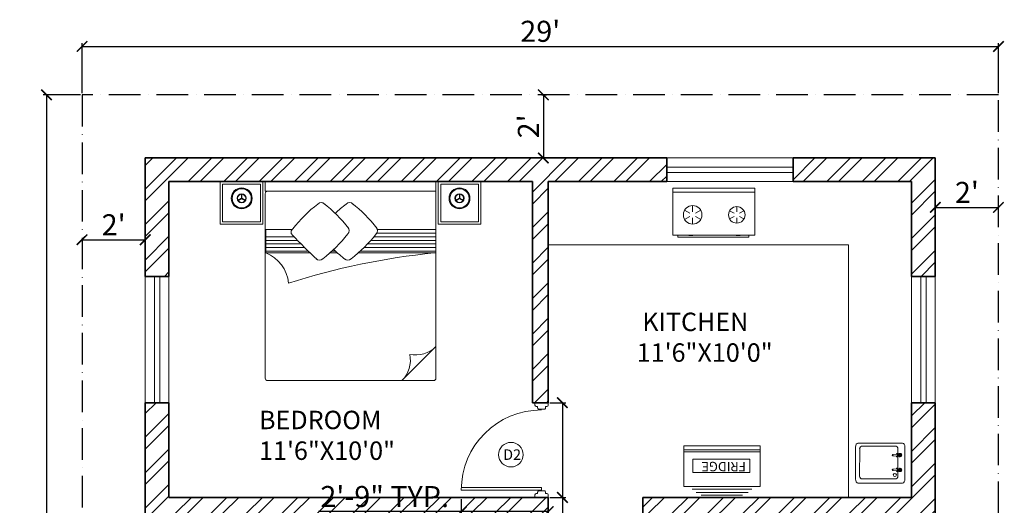
# Model space of a CAD drawing. Units: inches. Extents: x -15 to 1053, y -1 to 793.
# Tile 3 of 8: x 21 to 395, y 609 to 793. Entities that reach past the tile are written whole.
import ezdxf

# ---------------------------------------------------------------- set-up
doc = ezdxf.new("R2010")
doc.units = ezdxf.units.IN
doc.linetypes.add('ACAD_ISO10W100', pattern=[18, 12, -3, 0, -3])
for name, color, linetype, lineweight in [('00 FURNITURE', 15, 'Continuous', 15), ('A-ANNO-DIMS', 2, 'Continuous', 18), ('A-ANNO-TEXT', 7, 'Continuous', 18), ('A-AREA-IDEN', 7, 'Continuous', 18), ('A-DOOR', 4, 'Continuous', 18), ('A-FLOR-CASE', 5, 'Continuous', 18), ('A-FLOR-FIXT', 8, 'Continuous', 13), ('A-FURN', 8, 'Continuous', 13), ('A-GLAZ', 4, 'Continuous', 18), ('A-WALL', 7, 'Continuous', 35), ('A-WALL-PATT', 8, 'Continuous', 13), ('C-PROP', 1, 'ACAD_ISO10W100', 25)]:
    doc.layers.add(name, color=color, linetype=linetype, lineweight=lineweight)
doc.layers.add('FURN3D', color=229, linetype='Continuous', lineweight=5, true_color=0x4a3f41)
doc.layers.add('furniture', color=253, linetype='Continuous', lineweight=9, transparency=0.4)
doc.styles.add('1-100DIM', font='txt', dxfattribs={"height": 0.3})
doc.styles.get("Standard").update_dxf_attribs({"font": 'arial.ttf'})
doc.dimstyles.new('ISO-25', dxfattribs={"dimtxt": 8, "dimasz": 4, "dimexe": 1.25, "dimexo": 0.625, "dimtad": 1, "dimdec": 0, "dimlunit": 4, "dimtxsty": 'Standard', "dimblk": 'ARCHTICK', "dimcen": 3, "dimadec": 0, "dimazin": 0, "dimtfac": 1, "dimtdec": 0, "dimtmove": 0, "dimatfit": 3, "dimldrblk": 'ARCHTICK', "dimfxl": 1, "dimarcsym": 0})

# ---------------------------------------------------------------- blocks, each defined once
blk = doc.blocks.new('A$C21540130')
at = {"layer": 'FURN3D'}
for p, q in [((1.57, 0), (1.57, 31.11)), ((9.61, 25.31), (8.63, 27.01)), ((10.79, 25.31), (11.77, 27.01)), ((9.02, 24.29, -27.54), (7.06, 24.29, -27.54)), ((9.61, 23.27), (8.63, 21.57)), ((10.79, 23.27), (11.77, 21.57)), ((11.38, 24.29, -27.54), (13.34, 24.29, -27.54)), ((9.02, 7.54), (6.67, 7.54)), ((9.61, 8.56), (8.43, 10.6)), ((10.79, 8.56), (11.97, 10.6)), ((11.38, 7.54), (13.73, 7.54)), ((9.61, 6.52), (8.43, 4.48)), ((10.79, 6.52), (11.97, 4.48))]:
    blk.add_line(p, q, dxfattribs=at)
for points in [[(0, 0), (0, 31.11), (17.9, 31.11), (17.9, 0)], [(18.68, 1.96), (18.68, 28.83), (17.9, 28.83), (17.9, 1.96)]]:
    blk.add_lwpolyline(points, close=True, dxfattribs=at)
for centre, radius in [((10.2, 24.29), 3.14), ((10.2, 7.54), 3.53)]:
    blk.add_circle(centre, radius, dxfattribs=at)
for points in [[(17.9, 24.03), (18.29, 24.03), (17.9, 25.6), (18.29, 25.6)], [(17.9, 6.05), (18.29, 6.05), (17.9, 7.62), (18.29, 7.62)]]:
    blk.add_solid(points, dxfattribs=at)
blk = doc.blocks.new('A$C03CC5C65')
at = {"layer": 'FURN3D'}
for p, q in [((1.56, 18.72, -49.92), (13.66, 18.72, -49.92)), ((0, 0.9, -49.92), (0, 17.82, -49.92)), ((0, 0.9, -29.27), (0, 17.82, -48.65)), ((0, 17.82, -29.27), (0, 0.9, -48.65)), ((4.37, 16.77, -25.9), (4.37, 16.84, -25.9)), ((4.37, 16.77, -25.9), (4.73, 16.4, -25.9)), ((4.37, 15.7, -25.9), (4.73, 16.12, -25.9)), ((4.37, 15.64, -25.9), (4.73, 16.06, -25.9)), ((4.37, 15.64, -25.9), (4.37, 15.7, -25.9)), ((4.48, 16.95, -25.9), (4.87, 16.59, -25.9)), ((4.48, 16.89, -25.9), (4.48, 16.95, -25.9)), ((4.48, 16.89, -25.9), (4.87, 16.52, -25.9)), ((4.48, 15.53, -25.9), (4.87, 15.89, -25.9)), ((4.63, 16.87, -25.9), (4.63, 16.8, -25.9)), ((4.63, 15.67, -25.9), (4.68, 15.67, -25.9)), ((4.63, 15.67), (4.68, 15.67)), ((4.64, 16.49, -25.9), (4.66, 16.05, -25.9)), ((4.83, 16.98, -25.9), (4.68, 16.76, -25.9)), ((4.68, 15.71, -25.9), (4.75, 14.17, -25.9)), ((4.87, 16.91, -25.9), (4.73, 16.71, -25.9)), ((5.24, 16.98, -25.9), (4.83, 16.98, -25.9)), ((4.87, 16.91, -25.9), (4.83, 16.98, -25.9)), ((5.21, 16.91, -25.9), (4.87, 16.91, -25.9)), ((5.21, 16.91, -25.9), (5.24, 16.98, -25.9)), ((5.6, 16.95, -25.9), (5.21, 16.59, -25.9)), ((5.21, 16.91, -25.9), (5.34, 16.71, -25.9)), ((5.6, 16.88, -25.9), (5.21, 16.52, -25.9)), ((5.6, 15.52, -25.9), (5.21, 15.89, -25.9)), ((5.24, 16.98, -25.9), (5.39, 16.76, -25.9)), ((5.39, 15.71, -25.9), (5.32, 14.17, -25.9)), ((5.71, 16.77, -25.9), (5.35, 16.4, -25.9)), ((5.71, 15.7, -25.9), (5.35, 16.12, -25.9)), ((5.71, 15.64, -25.9), (5.35, 16.06, -25.9)), ((5.39, 15.67, -25.9), (5.44, 15.67, -25.9)), ((5.39, 15.67), (5.44, 15.67)), ((5.43, 16.49, -25.9), (5.41, 16.05, -25.9)), ((5.44, 16.87, -25.9), (5.44, 16.8, -25.9)), ((5.6, 16.95, -25.9), (5.6, 16.88, -25.9)), ((5.6, 16.95, -25.9), (5.6, 16.88, -25.9)), ((5.71, 16.77, -25.9), (5.71, 16.83, -25.9)), ((5.71, 15.64, -25.9), (5.71, 15.7, -25.9)), ((9.98, 15.69, -25.9), (10.34, 16.11, -25.9)), ((9.98, 15.63, -25.9), (10.34, 16.05, -25.9)), ((9.98, 15.63, -25.9), (9.98, 15.69, -25.9)), ((9.99, 16.76, -25.9), (9.99, 16.83, -25.9)), ((9.99, 16.76, -25.9), (10.34, 16.39, -25.9)), ((10.09, 16.94, -25.9), (10.48, 16.58, -25.9)), ((10.09, 16.88, -25.9), (10.09, 16.94, -25.9)), ((10.09, 16.88, -25.9), (10.48, 16.51, -25.9)), ((10.09, 15.52, -25.9), (10.48, 15.88, -25.9)), ((10.25, 16.86, -25.9), (10.25, 16.8, -25.9)), ((10.25, 15.66, -25.9), (10.3, 15.66, -25.9)), ((10.25, 15.66), (10.3, 15.66)), ((10.26, 16.47, -25.9), (10.28, 16.03, -25.9)), ((10.45, 16.97, -25.9), (10.3, 16.75, -25.9)), ((10.3, 15.7, -25.9), (10.37, 14.16, -25.9)), ((10.49, 16.9, -25.9), (10.35, 16.7, -25.9)), ((10.86, 16.97, -25.9), (10.45, 16.97, -25.9)), ((10.49, 16.9, -25.9), (10.45, 16.97, -25.9)), ((10.82, 16.9, -25.9), (10.49, 16.9, -25.9)), ((10.82, 16.9, -25.9), (10.86, 16.97, -25.9)), ((11.22, 16.94, -25.9), (10.82, 16.58, -25.9)), ((10.82, 16.9, -25.9), (10.96, 16.7, -25.9)), ((11.22, 16.88, -25.9), (10.82, 16.51, -25.9)), ((11.21, 15.51, -25.9), (10.82, 15.88, -25.9)), ((10.86, 16.97, -25.9), (11.01, 16.75, -25.9)), ((11.01, 15.7, -25.9), (10.93, 14.16, -25.9)), ((11.32, 16.76, -25.9), (10.96, 16.39, -25.9)), ((11.32, 15.69, -25.9), (10.96, 16.11, -25.9)), ((11.32, 15.63, -25.9), (10.96, 16.05, -25.9)), ((11.01, 15.66, -25.9), (11.06, 15.66, -25.9)), ((11.01, 15.66), (11.06, 15.66)), ((11.05, 16.47, -25.9), (11.03, 16.03, -25.9)), ((11.06, 16.86, -25.9), (11.06, 16.8, -25.9)), ((11.22, 16.94, -25.9), (11.22, 16.88, -25.9)), ((11.22, 16.94, -25.9), (11.22, 16.88, -25.9)), ((11.32, 16.76, -25.9), (11.32, 16.83, -25.9)), ((11.32, 15.63, -25.9), (11.32, 15.69, -25.9)), ((15.22, 0.9, -29.27), (15.22, 17.82, -48.65)), ((15.22, 17.82, -29.27), (15.22, 0.9, -48.65)), ((1.56, 0, -28), (13.66, 0, -28))]:
    blk.add_line(p, q, dxfattribs=at)
at = {"layer": 'FURN3D', "elevation": -25.9}
for points in [[(1.61, 15.14), (1.62, 2.5)], [(4.66, 16.1), (2.57, 16.1)], [(10.28, 16.11), (5.41, 16.1)], [(13.12, 16.11), (11.03, 16.11)], [(14.1, 2.52), (14.09, 15.15)], [(2.58, 1.55), (13.13, 1.56)]]:
    blk.add_lwpolyline(points, dxfattribs=at)
at = {"layer": 'FURN3D'}
for centre, radius in [((3.1, 14.9, -25.9), 0.593), ((5.04, 16.22, -25.9), 0.218), ((5.04, 16.87), 0.203), ((5.04, 16.87, -25.9), 0.203), ((10.65, 16.22, -25.9), 0.218), ((10.65, 16.86), 0.203), ((10.65, 16.86, -25.9), 0.203)]:
    blk.add_circle(centre, radius, dxfattribs=at)
at = {"layer": 'FURN3D', "extrusion": (0, 0.814703, 0.579878)}
for centre, start, end in [((-1.56, -49.97, -13.7), 270, 0), ((-13.66, -49.97, -13.7), 180, 270), ((-1.56, -24.37, -16.24), 0, 90), ((-13.66, -24.37, -16.24), 90, 180)]:
    blk.add_arc(centre, 1.56, start, end, dxfattribs=at)
at = {"layer": 'FURN3D', "extrusion": (2.9e-15, -0.814703, 0.579878)}
for centre, start, end in [((1.56, -13.52, -31.49), 90, 180), ((1.56, -39.11, -28.95), 180, 270)]:
    blk.add_arc(centre, 1.56, start, end, dxfattribs=at)
at = {"layer": 'FURN3D', "extrusion": (-2.9e-15, -0.814703, 0.579878)}
for centre, start, end in [((13.66, -13.52, -31.49), 0, 90), ((13.66, -39.11, -28.95), 270, 0)]:
    blk.add_arc(centre, 1.56, start, end, dxfattribs=at)
at = {"layer": 'FURN3D'}
for centre, radius, start, end in [((2.6, 15.1, -25.9), 0.997, 88.2299, 182.3676), ((4.6, 16.73, -25.9), 0.252, 118.1078, 154.1122), ((4.6, 16.66, -25.9), 0.252, 118.1078, 154.1122), ((4.6, 15.75, -25.9), 0.252, 205.7141, 241.7184), ((5.04, 16.87, -25.9), 0.655, 359.2227, 180.6036), ((5.04, 16.88, -25.9), 0.655, 190.8582, 233.614), ((5.04, 16.87, -25.9), 0.406, 359.9131, 179.9131), ((4.54, 16.23, -25.9), 0.25, 317.2189, 42.6074), ((4.54, 16.29, -25.9), 0.25, 317.2189, 352.664), ((5.04, 16.6, -25.9), 0.312, 19.462, 160.6639), ((5.04, 16.24, -25.9), 0.218, 356.8132, 183.0131), ((5.04, 16.77, -25.9), 0.25, 227.2092, 312.6171), ((5.04, 16.71, -25.9), 0.25, 227.2092, 312.6171), ((5.04, 15.7, -25.9), 0.25, 47.2092, 132.6171), ((5.04, 16.44, -25.9), 0.187, 40.218, 139.6082), ((5.53, 16.23, -25.9), 0.25, 137.2189, 222.6074), ((5.53, 16.29, -25.9), 0.25, 187.1622, 222.6074), ((5.04, 16.88, -25.9), 0.655, 306.2123, 348.968), ((5.48, 16.72, -25.9), 0.252, 25.7141, 61.7184), ((5.48, 16.66, -25.9), 0.252, 25.7141, 61.7184), ((5.48, 15.75, -25.9), 0.252, 298.1078, 334.1122), ((10.21, 15.74, -25.9), 0.252, 205.7141, 241.7184), ((10.21, 16.72, -25.9), 0.252, 118.1078, 154.1122), ((10.21, 16.65, -25.9), 0.252, 118.1078, 154.1122), ((10.65, 16.86, -25.9), 0.655, 359.2227, 180.6036), ((10.65, 16.86, -25.9), 0.655, 190.8582, 233.614), ((10.65, 16.86, -25.9), 0.406, 359.9131, 179.9131), ((10.16, 16.22, -25.9), 0.25, 317.2189, 42.6074), ((10.16, 16.28, -25.9), 0.25, 317.2189, 352.664), ((10.66, 16.59, -25.9), 0.312, 19.462, 160.6639), ((10.65, 16.23, -25.9), 0.218, 356.8132, 183.0131), ((10.65, 16.7, -25.9), 0.25, 227.2092, 312.6171), ((10.65, 15.69, -25.9), 0.25, 47.2092, 132.6171), ((10.65, 16.76, -25.9), 0.25, 227.2092, 312.6171), ((10.65, 16.44, -25.9), 0.187, 40.218, 139.6082), ((11.15, 16.22, -25.9), 0.25, 137.2189, 222.6074), ((11.15, 16.28, -25.9), 0.25, 187.1622, 222.6074), ((10.65, 16.86, -25.9), 0.655, 306.2123, 348.968), ((11.1, 15.74, -25.9), 0.252, 298.1078, 334.1122), ((11.1, 16.72, -25.9), 0.252, 25.7141, 61.7184), ((11.1, 16.65, -25.9), 0.252, 25.7141, 61.7184), ((13.09, 15.11, -25.9), 0.997, 357.7426, 91.8802), ((5.04, 14.37, -25.9), 0.298, 194.8671, 343.5351), ((5.03, 14.18, -25.9), 0.281, 182.7661, 357.0602), ((10.65, 14.36, -25.9), 0.298, 194.8671, 343.5351), ((10.65, 14.17, -25.9), 0.281, 182.7661, 357.0602), ((2.61, 2.54, -25.9), 0.997, 177.7426, 271.8802), ((13.1, 2.55, -25.9), 0.997, 268.2299, 2.3676)]:
    blk.add_arc(centre, radius, start, end, dxfattribs=at)
blk = doc.blocks.new('RGWTG')
at = {"layer": '00 FURNITURE'}
for p, q in [((578.23, 3473.51), (577.36, 3475.01)), ((578.23, 3473.58), (577.36, 3472.08)), ((578.36, 3473.58), (577.49, 3475.09)), ((578.36, 3473.51), (577.49, 3472)), ((578.29, 3473.62), (580.03, 3473.62)), ((578.29, 3473.47), (580.03, 3473.47)), ((521.93, 3464.58), (509.03, 3451.68)), ((509.03, 3422.63), (509.03, 3463.68)), ((509.93, 3464.58), (566.4, 3464.58)), ((557.53, 3463.84), (557.53, 3464.49)), ((557.53, 3464.49), (566.4, 3464.49)), ((558.2, 3464.49), (558.2, 3435.82)), ((559.57, 3464.49), (559.57, 3437.25)), ((560.94, 3464.49), (560.94, 3438.58)), ((562.3, 3464.49), (562.3, 3439.83)), ((563.67, 3464.49), (563.67, 3440.99)), ((565.04, 3464.49), (565.04, 3442.08)), ((566.4, 3464.58), (580.98, 3464.58)), ((566.4, 3464.49), (566.4, 3442.08)), ((566.4, 3464.49), (566.4, 3463.84)), ((580.98, 3464.58), (580.98, 3416.72)), ((558.2, 3426.48), (558.2, 3425.04)), ((509.03, 3400.68), (509.03, 3422.63)), ((558.2, 3416.13), (558.2, 3399.95)), ((559.57, 3414.75), (559.57, 3399.95)), ((580.98, 3416.72), (580.98, 3400.68)), ((560.94, 3413.39), (560.94, 3399.95)), ((562.3, 3412.04), (562.3, 3399.95)), ((563.67, 3410.72), (563.67, 3399.95)), ((580.08, 3399.78), (509.93, 3399.78)), ((557.53, 3399.95), (557.53, 3400.6)), ((566.4, 3399.95), (557.53, 3399.95)), ((566.4, 3400.6), (566.4, 3399.95)), ((578.23, 3390.78), (577.36, 3392.29)), ((578.36, 3390.86), (577.49, 3392.36)), ((578.23, 3390.86), (577.36, 3389.36)), ((578.36, 3390.78), (577.49, 3389.28)), ((578.29, 3390.9), (580.03, 3390.9)), ((578.29, 3390.74), (580.03, 3390.74))]:
    blk.add_line(p, q, dxfattribs=at)
for points in [[(568.43, 3465.48), (584.63, 3465.48), (584.63, 3481.68), (568.43, 3481.68)], [(569.33, 3466.38), (583.73, 3466.38), (583.73, 3480.78), (569.33, 3480.78)], [(580.98, 3399.78), (584.63, 3399.78), (584.63, 3464.58), (580.98, 3464.58)], [(568.43, 3398.88), (584.63, 3398.88), (584.63, 3382.68), (568.43, 3382.68)], [(569.33, 3397.98), (583.73, 3397.98), (583.73, 3383.58), (569.33, 3383.58)]]:
    blk.add_lwpolyline(points, close=True, dxfattribs=at)
for points in [[(566.52, 3464.49), (557.53, 3464.49), (557.53, 3435.08)], [(557.53, 3427.21), (557.53, 3424.3)], [(557.53, 3416.82), (557.53, 3399.95), (566.4, 3399.95), (566.4, 3409.94)]]:
    blk.add_lwpolyline(points, dxfattribs=at)
for centre, radius in [((578.29, 3473.54), 3.97), ((578.29, 3473.54), 3.63), ((578.29, 3473.54), 1.74), ((578.29, 3473.54), 1.56), ((578.29, 3390.82), 3.97), ((578.29, 3390.82), 3.63), ((578.29, 3390.82), 1.74), ((578.29, 3390.82), 1.56)]:
    blk.add_circle(centre, radius, dxfattribs=at)
for centre, radius, start, end in [((509.93, 3463.68), 0.9, 90, 180), ((529.65, 3456.88), 10.9, 135.0361, 191.9278), ((290.56, 3490.52), 268.3, 342.2214, 354.2925), ((516.73, 3443.97), 10.9, 78.0722, 134.9639), ((598.15, 3399.01), 54.32, 127.931, 142.069), ((566.05, 3440.57), 1.82, 45, 135), ((533.58, 3399.31), 54.32, 37.931, 52.069), ((556.59, 3431.11), 1.82, 135, 225), ((574.84, 3431.77), 1.82, 315, 45), ((597.87, 3463.6), 54.32, 217.931, 224.141), ((598.15, 3388.23), 54.32, 127.931, 142.069), ((566.05, 3429.78), 1.82, 45, 135), ((533.58, 3388.53), 54.32, 37.931, 52.069), ((533.28, 3463.88), 54.32, 316.32, 322.069), ((556.59, 3420.33), 1.82, 135, 225), ((574.84, 3420.99), 1.82, 315, 45), ((765.33, 3619.75), 290.45, 223.6069, 226.2326), ((533.28, 3453.1), 54.32, 307.931, 322.069), ((565.44, 3411.05), 1.47, 225.9674, 326.8337), ((545.02, 3395.29), 13.35, 20.4224, 85.5825), ((509.93, 3400.68), 0.9, 180, 270), ((580.08, 3400.68), 0.9, 270, 0)]:
    blk.add_arc(centre, radius, start, end, dxfattribs=at)
blk = doc.blocks.new('DDD')
at = {"layer": '00 FURNITURE'}
for p, q in [((-12579.77, -15859.53), (-12579.77, -15829.05)), ((-12578.77, -15859.53), (-12578.77, -15829.03)), ((-12612.02, -15857.03), (-12612.02, -15862.03)), ((-12611.02, -15857.03), (-12612.02, -15857.03)), ((-12610.52, -15858.03), (-12610.52, -15857.53)), ((-12578.77, -15859.53), (-12579.77, -15859.53)), ((-12577.52, -15858.03), (-12577.52, -15857.53)), ((-12577.02, -15857.03), (-12576.02, -15857.03)), ((-12576.02, -15857.03), (-12576.02, -15862.03)), ((-12612.02, -15862.03), (-12611.02, -15862.03)), ((-12610.52, -15861.53), (-12610.52, -15861.03)), ((-12577.52, -15861.53), (-12577.52, -15861.03)), ((-12576.02, -15862.03), (-12577.02, -15862.03))]:
    blk.add_line(p, q, dxfattribs=at)
for points in [[(-12610.52, -15861.03), (-12610.02, -15861.03, 0.414214), (-12609.52, -15860.53), (-12609.52, -15858.53, 0.414214), (-12610.02, -15858.03), (-12610.52, -15858.03)], [(-12577.52, -15861.03), (-12578.02, -15861.03, -0.414214), (-12578.52, -15860.53), (-12578.52, -15858.53, -0.414214), (-12578.02, -15858.03), (-12577.52, -15858.03)]]:
    blk.add_lwpolyline(points, format="xyb", dxfattribs=at)
for centre, radius, start, end in [((-12578.77, -15859.53), 30.5, 90, 180), ((-12611.02, -15857.53), 0.5, 0, 90), ((-12577.02, -15857.53), 0.5, 90, 180), ((-12611.02, -15861.53), 0.5, 270, 0), ((-12577.02, -15861.53), 0.5, 180, 270)]:
    blk.add_arc(centre, radius, start, end, dxfattribs=at)
blk = doc.blocks.new('A$C5BBA3387')
at = {"layer": 'furniture'}
for p, q in [((16.49, 29.07), (16.49, 0)), ((17.22, 29.07), (17.22, 0)), ((0, 22.44), (0, 6.75)), ((1.08, 24.37), (1.08, 4.58)), ((2.29, 25.81), (2.29, 3.26))]:
    blk.add_line(p, q, dxfattribs=at)
for points in [[(18.78, 29.07), (18.78, 0), (3.37, 0), (3.37, 29.07)], [(8.63, 4.02), (8.63, 25.56), (13.78, 25.56), (13.78, 4.02)]]:
    blk.add_lwpolyline(points, close=True, dxfattribs=at)
at = {"layer": 'furniture', "insert": (9.12, 5.47), "char_height": 3.589, "width": 57.8029, "attachment_point": 1, "rotation": 90}
blk.add_mtext('FRIDGE', dxfattribs=at)
blk = doc.blocks.new('_ArchTick')
at = {"color": 0, "linetype": 'ByBlock', "const_width": 0.15}
blk.add_lwpolyline([(-0.5, -0.5), (0.5, 0.5)], dxfattribs=at)
blk = doc.blocks.new('*D16')
at = {"layer": 'A-ANNO-DIMS', "color": 0, "lineweight": -2, "transparency": 16777216}
for p, q in [((44.87, 765.39), (44.87, 784.39)), ((44.87, 783.14), (392.87, 783.14)), ((392.87, 765.39), (392.87, 784.39))]:
    blk.add_line(p, q, dxfattribs=at)
at = {"layer": 'Defpoints', "color": 0, "transparency": 16777216}
for p in [(392.87, 783.14), (44.87, 764.76), (392.87, 764.76)]:
    blk.add_point(p, dxfattribs=at)
at = {"layer": 'A-ANNO-DIMS', "color": 0, "lineweight": -2, "transparency": 16777216, "xscale": 4, "yscale": 4, "zscale": 4, "rotation": 180}
blk.add_blockref('_ArchTick', (44.87, 783.14), dxfattribs=at)
at = {"layer": 'A-ANNO-DIMS', "color": 0, "lineweight": -2, "transparency": 16777216, "xscale": 4, "yscale": 4, "zscale": 4}
blk.add_blockref('_ArchTick', (392.87, 783.14), dxfattribs=at)
at = {"layer": 'A-ANNO-DIMS', "color": 0, "transparency": 16777216, "insert": (218.87, 787.85), "char_height": 8, "attachment_point": 5}
blk.add_mtext("29'", dxfattribs=at)
blk = doc.blocks.new('*D17')
at = {"layer": 'A-ANNO-DIMS', "color": 0, "lineweight": -2, "transparency": 16777216}
for p, q in [((44.24, 764.76), (30.11, 764.76)), ((31.36, 764.76), (31.36, 44.76)), ((44.24, 44.76), (30.11, 44.76))]:
    blk.add_line(p, q, dxfattribs=at)
at = {"layer": 'Defpoints', "color": 0, "transparency": 16777216}
for p in [(44.87, 764.76), (31.36, 44.76), (44.87, 44.76)]:
    blk.add_point(p, dxfattribs=at)
at = {"layer": 'A-ANNO-DIMS', "color": 0, "lineweight": -2, "transparency": 16777216, "xscale": 4, "yscale": 4, "zscale": 4}
for p, rotation in [((31.36, 764.76), 90), ((31.36, 44.76), 270)]:
    blk.add_blockref('_ArchTick', p, dxfattribs=dict(at, rotation=rotation))
at = {"layer": 'A-ANNO-DIMS', "color": 0, "transparency": 16777216, "insert": (26.65, 404.76), "char_height": 8, "attachment_point": 5, "rotation": 90}
blk.add_mtext("60'", dxfattribs=at)
blk = doc.blocks.new('*D25')
at = {"layer": 'A-ANNO-DIMS', "color": 0, "lineweight": -2, "transparency": 16777216}
for p, q in [((44.87, 710.17), (44.87, 708.43)), ((44.87, 709.68), (68.87, 709.68)), ((68.87, 710.17), (68.87, 708.43))]:
    blk.add_line(p, q, dxfattribs=at)
at = {"layer": 'Defpoints', "color": 0, "transparency": 16777216}
for p in [(44.87, 710.79), (68.87, 710.79), (68.87, 709.68)]:
    blk.add_point(p, dxfattribs=at)
at = {"layer": 'A-ANNO-DIMS', "color": 0, "lineweight": -2, "transparency": 16777216, "xscale": 4, "yscale": 4, "zscale": 4, "rotation": 180}
blk.add_blockref('_ArchTick', (44.87, 709.68), dxfattribs=at)
at = {"layer": 'A-ANNO-DIMS', "color": 0, "lineweight": -2, "transparency": 16777216, "xscale": 4, "yscale": 4, "zscale": 4}
blk.add_blockref('_ArchTick', (68.87, 709.68), dxfattribs=at)
at = {"layer": 'A-ANNO-DIMS', "color": 0, "transparency": 16777216, "insert": (56.87, 714.32), "char_height": 8, "attachment_point": 5}
blk.add_mtext("2'", dxfattribs=at)
blk = doc.blocks.new('*D26')
at = {"layer": 'A-ANNO-DIMS', "color": 0, "lineweight": -2, "transparency": 16777216}
for p, q in [((219.49, 764.76), (221.29, 764.76)), ((220.04, 764.76), (220.04, 740.76)), ((219.49, 740.76), (221.29, 740.76))]:
    blk.add_line(p, q, dxfattribs=at)
at = {"layer": 'Defpoints', "color": 0, "transparency": 16777216}
for p in [(218.87, 764.76), (218.87, 740.76), (220.04, 740.76)]:
    blk.add_point(p, dxfattribs=at)
at = {"layer": 'A-ANNO-DIMS', "color": 0, "lineweight": -2, "transparency": 16777216, "xscale": 4, "yscale": 4, "zscale": 4}
for p, rotation in [((220.04, 764.76), 90), ((220.04, 740.76), 270)]:
    blk.add_blockref('_ArchTick', p, dxfattribs=dict(at, rotation=rotation))
at = {"layer": 'A-ANNO-DIMS', "color": 0, "transparency": 16777216, "insert": (215.4, 752.76), "char_height": 8, "attachment_point": 5, "rotation": 90}
blk.add_mtext("2'", dxfattribs=at)
blk = doc.blocks.new('*D27')
at = {"layer": 'A-ANNO-DIMS', "color": 0, "lineweight": -2, "transparency": 16777216}
for p, q in [((368.87, 721.91), (368.87, 723.23)), ((368.87, 721.98), (392.87, 721.98)), ((392.87, 721.91), (392.87, 723.23))]:
    blk.add_line(p, q, dxfattribs=at)
at = {"layer": 'Defpoints', "color": 0, "transparency": 16777216}
for p in [(392.87, 721.98), (368.87, 721.28), (392.87, 721.28)]:
    blk.add_point(p, dxfattribs=at)
at = {"layer": 'A-ANNO-DIMS', "color": 0, "lineweight": -2, "transparency": 16777216, "xscale": 4, "yscale": 4, "zscale": 4, "rotation": 180}
blk.add_blockref('_ArchTick', (368.87, 721.98), dxfattribs=at)
at = {"layer": 'A-ANNO-DIMS', "color": 0, "lineweight": -2, "transparency": 16777216, "xscale": 4, "yscale": 4, "zscale": 4}
blk.add_blockref('_ArchTick', (392.87, 721.98), dxfattribs=at)
at = {"layer": 'A-ANNO-DIMS', "color": 0, "transparency": 16777216, "insert": (380.87, 726.62), "char_height": 8, "attachment_point": 5}
blk.add_mtext("2'", dxfattribs=at)
blk = doc.blocks.new('*D34')
at = {"layer": 'A-ANNO-DIMS', "color": 0, "lineweight": -2, "transparency": 16777216}
for p, q in [((222.49, 647.76), (228.52, 647.76)), ((227.27, 647.76), (227.27, 611.76)), ((222.49, 611.76), (228.52, 611.76)), ((227.27, 611.76), (227.27, 521.52))]:
    blk.add_line(p, q, dxfattribs=at)
at = {"layer": 'Defpoints', "color": 0, "transparency": 16777216}
for p in [(221.87, 647.76), (221.87, 611.76), (227.27, 611.76)]:
    blk.add_point(p, dxfattribs=at)
at = {"layer": 'A-ANNO-DIMS', "color": 0, "lineweight": -2, "transparency": 16777216, "xscale": 4, "yscale": 4, "zscale": 4}
for p, rotation in [((227.27, 647.76), 90), ((227.27, 611.76), 270)]:
    blk.add_blockref('_ArchTick', p, dxfattribs=dict(at, rotation=rotation))
at = {"layer": 'A-ANNO-DIMS', "color": 0, "transparency": 16777216, "insert": (222.5, 564.64), "char_height": 8, "attachment_point": 5, "rotation": 90}
blk.add_mtext('DOOR 3\'-0" TYP.', dxfattribs=at)
blk = doc.blocks.new('*D35')
at = {"layer": 'A-ANNO-DIMS', "color": 0, "lineweight": -2, "transparency": 16777216}
for p, q in [((188.87, 611.14), (188.87, 605.11)), ((221.87, 611.14), (221.87, 605.11)), ((188.87, 606.36), (134.72, 606.36)), ((221.87, 606.36), (188.87, 606.36))]:
    blk.add_line(p, q, dxfattribs=at)
at = {"layer": 'Defpoints', "color": 0, "transparency": 16777216}
for p in [(188.87, 611.76), (221.87, 611.76), (188.87, 606.36)]:
    blk.add_point(p, dxfattribs=at)
at = {"layer": 'A-ANNO-DIMS', "color": 0, "lineweight": -2, "transparency": 16777216, "xscale": 4, "yscale": 4, "zscale": 4, "rotation": 180}
blk.add_blockref('_ArchTick', (188.87, 606.36), dxfattribs=at)
at = {"layer": 'A-ANNO-DIMS', "color": 0, "lineweight": -2, "transparency": 16777216, "xscale": 4, "yscale": 4, "zscale": 4}
blk.add_blockref('_ArchTick', (221.87, 606.36), dxfattribs=at)
at = {"layer": 'A-ANNO-DIMS', "color": 0, "transparency": 16777216, "insert": (159.79, 611.07), "char_height": 8, "attachment_point": 5}
blk.add_mtext('2\'-9" TYP.', dxfattribs=at)

msp = doc.modelspace()

# ---------------------------------------------------------------- hatches: boundary and pattern name
at = {"layer": 'A-WALL-PATT'}
h = msp.add_hatch(dxfattribs=at)
h.set_pattern_fill('ANSI32', color=256)
h.paths.add_polyline_path([(266.87, 740.76), (68.87, 740.76), (68.87, 695.76), (77.87, 695.76), (77.87, 731.76), (215.87, 731.76), (215.87, 647.76), (221.87, 647.76), (221.87, 731.76), (266.87, 731.76)])
h.paths.add_polyline_path([(368.87, 740.76), (314.87, 740.76), (314.87, 731.76), (359.87, 731.76), (359.87, 695.76), (368.87, 695.76)])
h.paths.add_polyline_path([(368.87, 647.76), (359.87, 647.76), (359.87, 611.76), (257.87, 611.76), (257.87, 605.76), (281.87, 605.76), (281.87, 587.76), (287.87, 587.76), (287.87, 605.76), (359.87, 605.76), (359.87, 593.76), (368.87, 593.76)])
h.paths.add_polyline_path([(245.87, 377.76), (221.87, 377.76), (221.87, 611.76), (216.87, 611.76), (77.87, 611.76), (77.87, 647.76), (68.87, 647.76), (68.87, 605.76), (215.87, 605.76), (215.87, 475.76), (191.87, 475.76), (191.87, 469.76), (215.87, 469.76), (215.87, 368.76), (245.87, 368.76)])
h.paths.add_polyline_path([(368.87, 503.76), (359.87, 503.76), (359.87, 368.76), (368.87, 368.76)])
h.paths.add_polyline_path([(368.87, 569.76), (359.87, 569.76), (359.87, 557.76), (257.87, 557.76), (257.87, 551.76), (368.87, 551.76)])
h.paths.add_polyline_path([(155.87, 475.76), (77.87, 475.76), (77.87, 569.76), (68.87, 569.76), (68.87, 469.76), (155.87, 469.76)])
h.paths.add_polyline_path([(77.87, 319.76), (179.87, 319.76), (179.87, 325.76), (77.87, 325.76), (77.87, 421.76), (68.87, 421.76), (68.87, 308.26), (77.87, 308.26)])
h.paths.add_polyline_path([(77.87, 266.76), (179.87, 266.76), (179.87, 272.76), (155.87, 272.76), (155.87, 289.76), (149.87, 289.76), (149.87, 272.76), (77.87, 272.76), (77.87, 284.26), (68.87, 284.26), (68.87, 230.76), (77.87, 230.76)], flags=17)
h.paths.add_polyline_path([(224.87, 326.76), (215.87, 326.76), (215.87, 146.76), (77.87, 146.76), (77.87, 182.76), (68.87, 182.76), (68.87, 146.76), (44.87, 146.76), (44.87, 44.76), (224.87, 44.76), (224.87, 53.76), (53.87, 53.76), (53.87, 137.76), (224.87, 137.76)])

# ---------------------------------------------------------------- linework, layer by layer
at = {"layer": 'A-ANNO-TEXT'}
msp.add_circle((207.73, 628.01), 4.67, dxfattribs=at)
at = {"layer": 'A-FLOR-CASE'}
for p, q in [((335.87, 707.76), (221.87, 707.76)), ((335.87, 611.76), (335.87, 707.76))]:
    msp.add_line(p, q, dxfattribs=at)
at = {"layer": 'A-GLAZ'}
for p, q in [((314.87, 740.76), (266.87, 740.76)), ((314.87, 737.26), (266.87, 737.26)), ((314.87, 735.26), (266.87, 735.26)), ((314.87, 731.76), (266.87, 731.76)), ((68.87, 695.76), (68.87, 647.76)), ((72.37, 695.76), (72.37, 647.76)), ((74.37, 695.76), (74.37, 647.76)), ((77.87, 695.76), (77.87, 647.76)), ((359.87, 695.76), (359.87, 647.76)), ((363.37, 695.76), (363.37, 647.76)), ((365.37, 695.76), (365.37, 647.76)), ((368.87, 695.76), (368.87, 647.76))]:
    msp.add_line(p, q, dxfattribs=at)
at = {"layer": 'A-WALL'}
for p, q in [((68.87, 740.76), (68.87, 695.76)), ((266.87, 740.76), (68.87, 740.76)), ((266.87, 731.76), (266.87, 740.76)), ((368.87, 740.76), (314.87, 740.76)), ((314.87, 731.76), (314.87, 740.76)), ((368.87, 695.76), (368.87, 740.76)), ((77.87, 731.76), (77.87, 695.76)), ((215.87, 731.76), (77.87, 731.76)), ((215.87, 731.76), (215.87, 647.76)), ((221.87, 731.76), (221.87, 647.76)), ((266.87, 731.76), (221.87, 731.76)), ((359.87, 731.76), (314.87, 731.76)), ((359.87, 695.76), (359.87, 731.76)), ((77.87, 695.76), (68.87, 695.76)), ((359.87, 695.76), (368.87, 695.76)), ((77.87, 647.76), (68.87, 647.76)), ((68.87, 647.76), (68.87, 605.76)), ((77.87, 647.76), (77.87, 611.76)), ((221.87, 647.76), (215.87, 647.76)), ((359.87, 611.76), (359.87, 647.76)), ((359.87, 647.76), (368.87, 647.76)), ((368.87, 593.76), (368.87, 647.76)), ((221.87, 611.76), (77.87, 611.76)), ((221.87, 611.76), (221.87, 377.76)), ((359.87, 611.76), (257.87, 611.76)), ((257.87, 611.76), (257.87, 605.76))]:
    msp.add_line(p, q, dxfattribs=at)
at = {"layer": 'C-PROP'}
for p, q in [((392.87, 764.76), (44.87, 764.76)), ((44.87, 764.76), (44.87, 44.76)), ((392.87, 44.76), (392.87, 764.76))]:
    msp.add_line(p, q, dxfattribs=at)

# ---------------------------------------------------------------- block references
at = {"layer": 'A-DOOR', "xscale": -1, "rotation": 90}
msp.add_blockref('DDD', (-15640.16, -11964.26), dxfattribs=at)
at = {"layer": 'A-DOOR', "rotation": 90}
msp.add_blockref('A$C5BBA3387', (302.41, 612.57), dxfattribs=at)
at = {"layer": 'A-FLOR-FIXT', "rotation": 270}
msp.add_blockref('A$C21540130', (269.2, 729.34), dxfattribs=at)
at = {"layer": 'A-FLOR-FIXT', "xscale": -1, "rotation": 270}
msp.add_blockref('A$C03CC5C65', (338.6, 617.19, 49.92), dxfattribs=at)
at = {"layer": 'A-FURN', "xscale": -1, "rotation": 270}
msp.add_blockref('RGWTG', (-3285.32, 147.13), dxfattribs=at)

# ---------------------------------------------------------------- texts
at = {"layer": 'A-ANNO-TEXT', "insert": (204.79, 630.03), "char_height": 4, "attachment_point": 1}
msp.add_mtext_dynamic_manual_height_columns('D2', width=8.4888, gutter_width=12.5, heights=[0], dxfattribs=at)
at = {"layer": 'A-AREA-IDEN', "char_height": 7, "attachment_point": 1, "style": '1-100DIM'}
for s, width, insert in [('{\\f@Malgun Gothic|b0|i0|c0|p34;   KITCHEN\\P  11\'6"X10\'0"}', 99.7063, (251.2, 681.98)), ('{\\f@Malgun Gothic|b0|i0|c0|p34;BEDROOM  11\'6"X10\'0"}', 54.0094, (112.08, 644.7))]:
    msp.add_mtext_dynamic_manual_height_columns(s, width=width, gutter_width=15.85, heights=[0], dxfattribs=dict(at, insert=insert))

# ---------------------------------------------------------------- dimensions: what is measured, and where the dimension line sits
at = {"layer": 'A-ANNO-DIMS'}
for base, p1, p2, picture, middle in [((392.87, 783.14), (44.87, 764.76), (392.87, 764.76), '*D16', (218.87, 787.85)), ((392.87, 721.98), (368.87, 721.28), (392.87, 721.28), '*D27', (380.87, 726.62)), ((68.87, 709.68), (44.87, 710.79), (68.87, 710.79), '*D25', (56.87, 714.32))]:
    dim = msp.add_linear_dim(base=base, p1=p1, p2=p2, dimstyle='ISO-25', override={"dimclrd": 0, "dimclre": 0, "dimclrt": 0}, dxfattribs=at)
    dim.commit()
    dim.dimension.update_dxf_attribs({"geometry": picture, "text_midpoint": middle})
for base, p1, p2, picture, middle in [((31.36, 44.76), (44.87, 764.76), (44.87, 44.76), '*D17', (26.65, 404.76)), ((220.04, 740.76), (218.87, 764.76), (218.87, 740.76), '*D26', (215.4, 752.76))]:
    dim = msp.add_linear_dim(base=base, p1=p1, p2=p2, angle=90, dimstyle='ISO-25', override={"dimclrd": 0, "dimclre": 0, "dimclrt": 0}, dxfattribs=at)
    dim.commit()
    dim.dimension.update_dxf_attribs({"geometry": picture, "text_midpoint": middle})
for base, p1, p2, angle, text, picture, middle in [((227.27, 611.76), (221.87, 647.76), (221.87, 611.76), 270, 'DOOR <> TYP.', '*D34', (222.5, 564.64)), ((188.87, 606.36), (221.87, 611.76), (188.87, 611.76), 180, '<> TYP.', '*D35', (159.79, 611.07))]:
    dim = msp.add_linear_dim(base=base, p1=p1, p2=p2, angle=angle, text=text, dimstyle='ISO-25', override={"dimdec": 1, "dimrnd": 0, "dimzin": 1, "dimlunit": 4, "dimfrac": 2}, dxfattribs=at)
    dim.commit()
    dim.dimension.update_dxf_attribs({"geometry": picture, "text_midpoint": middle})

doc.saveas('drawing.dxf')
